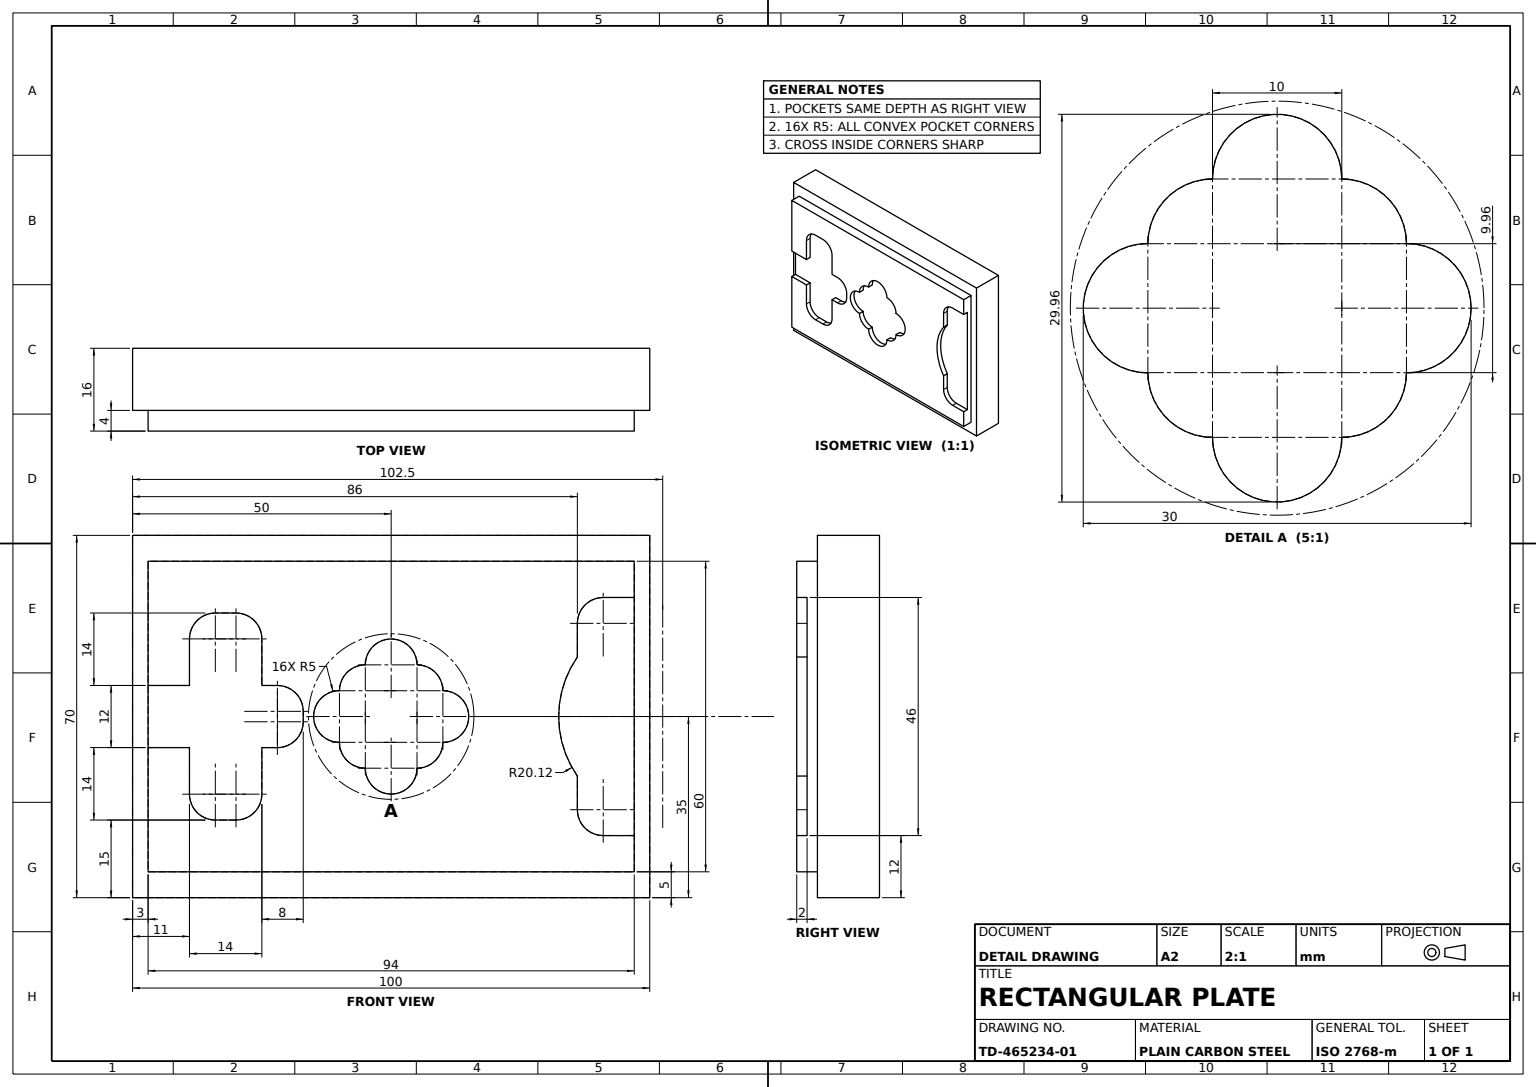
SolidWorks part; units mm, degrees
material "Plain Carbon Steel"
ref_plane "Front Plane" through (0, 0, 0) normal (0, 0, 1) x (1, 0, 0)
ref_plane "Top Plane" through (0, 0, 0) normal (0, 1, 0) x (1, 0, 0)
ref_plane "Right Plane" through (0, 0, 0) normal (1, 0, 0) x (0, 0, -1)
sketch "Base Plate Sketch" plane through (0, 0, 0) normal (0, 0, 1) x (1, 0, 0)
  line L1 (-50, 35) -> (50, 35)
  line L2 (-50, 35) -> (-50, -35)
  line L3 (-50, -35) -> (50, -35)
  line L4 (50, 35) -> (50, -35)
  line L5 (-50, 35) -> (50, -35) construction
  line L6 (-50, -35) -> (50, 35) construction
  point P0 (0, 0)
  dimension "D1" = 100
  dimension "D2" = 70
extrude "Base Plate 100x70x12" add sketch "Base Plate Sketch" along normal mid plane 12
sketch "Raised Pad Sketch" plane through (0, 0, -6) normal (0, 0, -1) x (-1, 0, 0)
  line L1 (47, 30) -> (-47, 30)
  line L2 (47, 30) -> (47, -30)
  line L3 (47, -30) -> (-47, -30)
  line L4 (-47, 30) -> (-47, -30)
  line L5 (47, 30) -> (-47, -30) construction
  line L6 (47, -30) -> (-47, 30) construction
  point P0 (0, 0)
  dimension "D1" = 94
  dimension "D2" = 60
extrude "Raised Pad 94x60x4" add sketch "Raised Pad Sketch" along normal blind 4
sketch "Pad Cut 1 Sketch" plane through (0, 0, -10) normal (0, 0, -1) x (-1, 0, 0)
  line L1 (47, -23) -> (47, 23)
  line L2 (47, -30) -> (47, 30) construction
  line L3 (47, -30) -> (47, 30) construction
  line L4 (-47, 30) -> (-47, -30) construction
  line L8 (-47, -30) -> (47, -30) construction
  line L9 (47, -30) -> (47, -23)
  line L10 (47, 23) -> (41, 23)
  line L11 (36, 18) -> (36, 11.5)
  line L12 (47, -23) -> (41, -23)
  line L13 (36, -18) -> (36, -11.5)
  arc A0 (41, -23) -> (36, -18) centre (41, -18) cw
  arc A1 (41, 23) -> (36, 18) centre (41, 18) ccw
  arc A2 (36, -11.5) -> (36, 11.5) centre (52.505, 0) cw
  point P17 (36, 0)
  dimension "D1" = 5
  dimension "D2" = 20.1163
  dimension "D3" = 83
  dimension "D4" = 99.505
  dimension "D5" = 7
  dimension "D6" = 18.5
extrude "Pad Cut 1" cut sketch "Pad Cut 1 Sketch" against normal mid plane 4 contours L12 A0 L13 A2 L11 A1 L10 L1
sketch "Pad Cut 2 Sketch" plane through (0, 0, -10) normal (0, 0, -1) x (-1, 0, 0)
  line L0 (-25, 0) -> (-17, 0)
  line L1 (36, -11.5) -> (36, -18) construction
  line L2 (-47, -6) -> (-39, -6)
  line L3 (-47, 6) -> (-39, 6)
  line L4 (-25, 6) -> (-22, 6)
  line L5 (-17, 1) -> (-17, -1.0106)
  line L6 (-34, 20) -> (-30, 20)
  line L7 (-34, -20) -> (-30, -20)
  line L8 (-22.0178, -6.0106) -> (-25, -6)
  line L9 (-47, -6) -> (-47, 6)
  line L10 (-25, 15) -> (-25, 6)
  line L11 (-39, 15) -> (-39, 6)
  line L12 (-25, -15) -> (-25, -6)
  line L13 (-39, -6) -> (-39, -15)
  line L14 (41, -23) -> (47, -23) construction
  arc A0 (-30, -20) -> (-25, -15) centre (-30, -15) ccw
  arc A1 (-34, -20) -> (-39, -15) centre (-34, -15) cw
  arc A2 (-30, 20) -> (-25, 15) centre (-30, 15) cw
  arc A3 (-34, 20) -> (-39, 15) centre (-34, 15) ccw
  arc A4 (-17, 1) -> (-22, 6) centre (-22, 1) ccw
  arc A5 (-17, -1.0106) -> (-22.0178, -6.0106) centre (-22, -1.0106) cw
  point P15 (-32, 20)
  point P18 (-32, -20)
  dimension "D1" = 5
  dimension "D3" = 5
  dimension "D4" = 53
  dimension "D5" = 58.0178
  dimension "D2" = 8
  dimension "D6" = 68
  dimension "D7" = 3
  dimension "D8" = 16.9894
  dimension "D9" = 29
extrude "Pad Cut 2" cut sketch "Pad Cut 2 Sketch" against normal mid plane 4 contours A3 L11 L3 L9 L2 L13 A1 L7 A0 L12 L8 A5 L5 A4 L4 L10 A2 L6
sketch "Pad Cut 3 Sketch" plane through (0, 0, -10) normal (0, 0, -1) x (-1, 0, 0)
  line L0 (0, 9.9824) -> (0, -9.9824)
  line L1 (-10, 0) -> (10, 0)
  line L2 (8.8, 0) -> (-8.8, 0) construction
  line L3 (0, 8.8) -> (0, -8.8) construction
  arc A0 (-10, 5) -> (-10, -5) centre (-10, 0) ccw
  arc A1 (5, 9.9824) -> (-5, 9.9824) centre (0, 9.9824) ccw
  arc A2 (10, -5) -> (10, 5) centre (10, 0) ccw
  arc A3 (-5, -9.9824) -> (5, -9.9824) centre (0, -9.9824) ccw
  arc A4 (-10, 5) -> (-5, 9.9824) centre (-5, 4.9824) cw
  arc A5 (-10, -5) -> (-5, -9.9824) centre (-5, -4.9824) ccw
  arc A6 (10, -5) -> (5, -9.9824) centre (5, -4.9824) cw
  arc A7 (10, 5) -> (5, 9.9824) centre (5, 4.9824) ccw
  point P4 (0, 0)
  point P8 (0, 0)
  dimension "D2" = 5
  dimension "D1" = 20
extrude "Pad Cut 3" cut sketch "Pad Cut 3 Sketch" against normal mid plane 4 contours A0 A5 A3 A6 A2 A7 A1 A4
